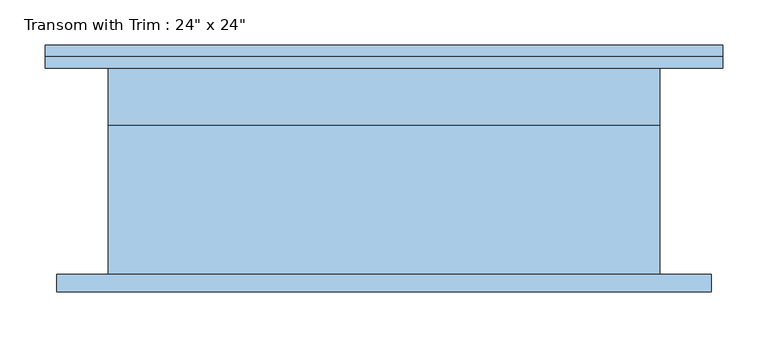
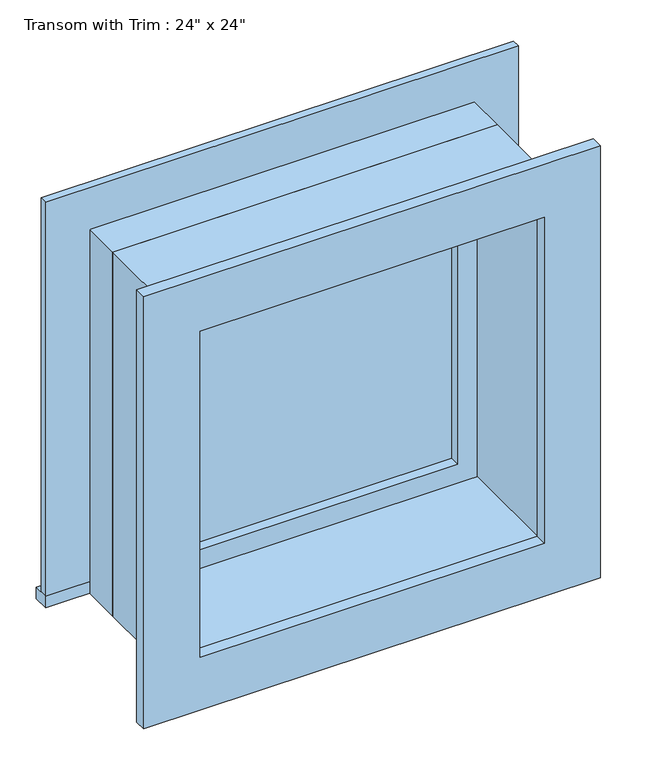
"""IFC4 building model written with IfcOpenShell, lengths in millimetres: window geometry."""

from ifc_helpers import new_model, si_unit, frame, origin, place, context, project, spatial, polyline, outline, extrude, source, transform, mapped, element, save


def window_3ed046d9(model_context):
    return source(origin(), model_context, "Body", "SweptSolid", [
        extrude(outline(polyline([(-412.75, 139.7), (336.55, 139.7), (336.55, 114.3), (-412.75, 114.3), (-412.75, 139.7)])), frame((0.0, 0.0, 2159.0), z_axis=(0.0, 0.0, 1.0), x_axis=(1.0, 0.0, 0.0)), (0.0, 0.0, 1.0), 19.05),
        extrude(outline(polyline([(2749.55, -323.85), (2749.55, 247.65), (2178.05, 247.65), (2178.05, 336.55), (2838.45, 336.55), (2838.45, -412.75), (2178.05, -412.75), (2178.05, -323.85), (2749.55, -323.85)])), frame((0.0, 114.3, 0.0), z_axis=(0.0, 1.0, 0.0), x_axis=(0.0, 0.0, 1.0)), (0.0, 0.0, 1.0), 12.7),
        extrude(outline(polyline([(2825.75, 323.85), (2825.75, -400.05), (2101.85, -400.05), (2101.85, 323.85), (2825.75, 323.85)]), holes=[polyline([(2736.85, 234.95), (2190.75, 234.95), (2190.75, -311.15), (2736.85, -311.15), (2736.85, 234.95)])]), frame((0.0, -133.35, 0.0), z_axis=(0.0, 1.0, 0.0), x_axis=(0.0, 0.0, 1.0)), (0.0, 0.0, 1.0), 19.05),
        extrude(outline(polyline([(203.2, 66.675), (-279.4, 66.675), (-279.4, 79.375), (203.2, 79.375), (203.2, 66.675)])), frame((0.0, 0.0, 2222.5), z_axis=(0.0, 0.0, 1.0), x_axis=(1.0, 0.0, 0.0)), (0.0, 0.0, 1.0), 482.6),
        extrude(outline(polyline([(2749.55, -323.85), (2178.05, -323.85), (2178.05, 247.65), (2749.55, 247.65), (2749.55, -323.85)]), holes=[polyline([(2705.1, -279.4), (2705.1, 203.2), (2222.5, 203.2), (2222.5, -279.4), (2705.1, -279.4)])]), frame((0.0, 50.8, 0.0), z_axis=(0.0, 1.0, 0.0), x_axis=(0.0, 0.0, 1.0)), (0.0, 0.0, 1.0), 44.45),
        extrude(outline(polyline([(2768.6, -342.9), (2159.0, -342.9), (2159.0, 266.7), (2768.6, 266.7), (2768.6, -342.9)]), holes=[polyline([(2736.85, -311.15), (2736.85, 234.95), (2190.75, 234.95), (2190.75, -311.15), (2736.85, -311.15)])]), frame((0.0, -114.3, 0.0), z_axis=(0.0, 1.0, 0.0), x_axis=(0.0, 0.0, 1.0)), (0.0, 0.0, 1.0), 165.1),
        extrude(outline(polyline([(2768.6, 266.7), (2768.6, -342.9), (2159.0, -342.9), (2159.0, 266.7), (2768.6, 266.7)]), holes=[polyline([(2749.55, 247.65), (2178.05, 247.65), (2178.05, -323.85), (2749.55, -323.85), (2749.55, 247.65)])]), frame((0.0, 50.8, 0.0), z_axis=(0.0, 1.0, 0.0), x_axis=(0.0, 0.0, 1.0)), (0.0, 0.0, 1.0), 63.5),
    ])


if __name__ == "__main__":
    model = new_model("IFC4")
    model_context = context("Model", 3, world=origin())
    ifc_project = project(units=[si_unit("LENGTHUNIT", "METRE", prefix="MILLI")], contexts=[model_context])
    site = spatial("IfcSite", under=ifc_project)
    building = spatial("IfcBuilding", under=site)
    placement = place(None, origin())
    window_shape = window_3ed046d9(model_context)
    element("IfcWindow", 1, ObjectType="Transom with Trim : 24\" x 24\"", at=placement, inside=building, context=model_context, shape_type="MappedRepresentation", body=[
        mapped(window_shape, transform((0.0, 0.0, 0.0), x_axis=(1.0, 0.0, 0.0), y_axis=(0.0, 1.0, 0.0), z_axis=(0.0, 0.0, 1.0))),
    ])
    save(model, "model.ifc")

# Revit data of these elements
# Type "Transom with Trim : 24\" x 24\""
#   Type Mark = "13"
#   Construction Type Id = "GSP4R"
#   Assembly Code = "B2020100"
#   Analytic Construction = "1/8 in Pilkington single glazing"
#   Visual Light Transmittance = 0.9
#   Solar Heat Gain Coefficient = 0.78
#   Heat Transfer Coefficient (U) = 0.6496 BTU/(h·ft²·°F)
#   Height = 2' - 0"
#   Default Sill Height = 7' - 1"
#   Trim Projection - Ext. = 0' - 0 1/2"
#   Trim Projection - Int. = 0' - 0 3/4"
#   Trim Width - Exterior = 0' - 3 1/2"
#   Trim Width - Interior = 0' - 3 1/2"
#   Width = 2' - 0"
#   Window Inset = 0' - 0 3/4"
#   Define Thermal Properties by = 1
#   Glass Pane Material = Glass
#   Sash Material = Sash
#   Trim Exterior Material = Trim
#   Trim Interior Material = Trim
#   Wall Closure = (empty or 0)
# Element 1 (IfcWindow, "Transom with Trim : 24\" x 24\"")
#   Materials on its faces: "Sash", "Trim", "Glass"
# Materials
#   "Glass": class "Glass", colour RGB 0 128 192, transparency 0.75, Description = "Soda Lime Glass", Cost = 0
#   "Sash": class "Wood", colour RGB 224 178 126, transparency 0
#   "Trim": class "Wood", colour RGB 224 178 126, transparency 0
